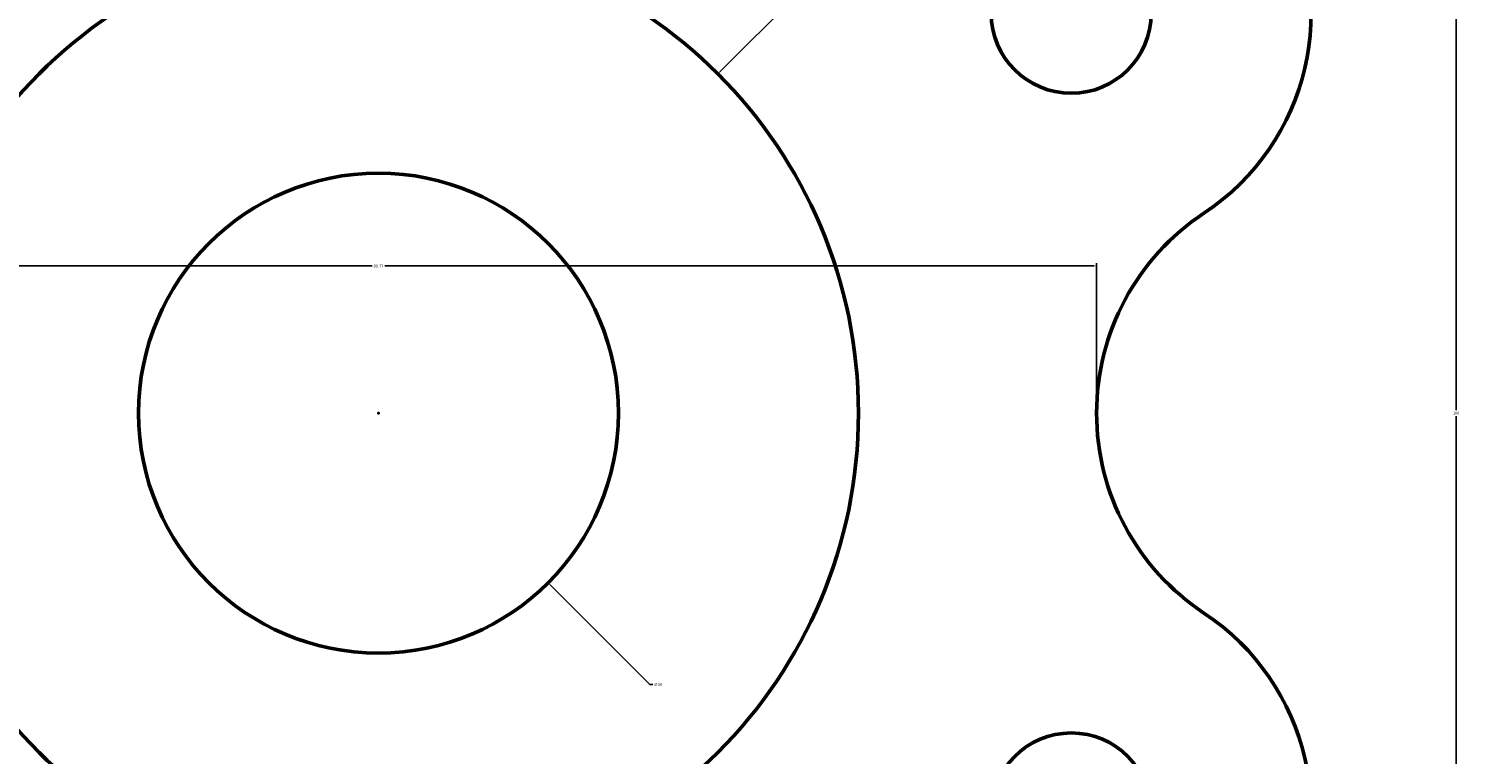
# Model space of a CAD drawing. Units: millimetres. Extents: x 2038 to 2173, y 1596 to 1745.
# Tile 3 of 4: x 2084 to 2173, y 1649 to 1695. Entities that reach past the tile are written whole.
import ezdxf

# ---------------------------------------------------------------- set-up
doc = ezdxf.new("R2010")
doc.units = ezdxf.units.MM
doc.layers.add('M-DIMS', color=2, linetype='Continuous', lineweight=18)
doc.layers.add('M-OUTL', color=7, linetype='Continuous', lineweight=50)
doc.styles.get("Standard").update_dxf_attribs({"font": 'arial.ttf'})
doc.dimstyles.get("Standard").update_dxf_attribs({"dimtxt": 0.18, "dimasz": 0.18, "dimexe": 0.18, "dimexo": 0.0625, "dimgap": 0.09, "dimtad": 0, "dimtih": 1, "dimtoh": 1, "dimdec": 4, "dimzin": 0, "dimdsep": 46, "dimtxsty": 'Standard', "dimcen": 0.09, "dimadec": 0, "dimazin": 0, "dimtfac": 1, "dimtdec": 4, "dimtofl": 0, "dimtmove": 0, "dimatfit": 3, "dimfxl": 1, "dimtolj": 1, "dimtzin": 0, "dimarcsym": 0})

# ---------------------------------------------------------------- blocks, each defined once
blk = doc.blocks.new('*U1')
blk.add_arc((-4.146, 7.965), 15, 243.55731, 356.44269)
blk = doc.blocks.new('*U2')
at = {"layer": 'M-OUTL', "color": 0, "linetype": 'ByBlock', "lineweight": -2, "transparency": 16777216, "rotation": 240}
blk.add_blockref('*U1', (2156.401, 1671.177), dxfattribs=at)
blk = doc.blocks.new('FLANGE-LUG-D10')
blk.add_circle((0, 0), 5)
blk.add_arc((0, 0), 15, 3.55731, 176.44269)
blk = doc.blocks.new('*D5')
at = {"layer": 'Defpoints', "color": 0, "transparency": 16777216}
for p in [(2038.131, 1735.784), (2105.488, 1735.784), (2105.488, 1605.784)]:
    blk.add_point(p, dxfattribs=at)
at = {"layer": 'M-DIMS', "color": 0, "lineweight": -2, "transparency": 16777216}
for p, q in [((2105.425, 1735.784), (2037.951, 1735.784)), ((2038.131, 1735.604), (2038.131, 1670.966)), ((2038.131, 1605.964), (2038.131, 1670.602)), ((2105.425, 1605.784), (2037.951, 1605.784))]:
    blk.add_line(p, q, dxfattribs=at)
at = {"layer": 'M-DIMS', "color": 0, "transparency": 16777216}
for points in [[(2038.101, 1735.604), (2038.161, 1735.604), (2038.131, 1735.784)], [(2038.101, 1605.964), (2038.161, 1605.964), (2038.131, 1605.784)]]:
    blk.add_solid(points, dxfattribs=at)
at = {"layer": 'M-DIMS', "color": 0, "transparency": 16777216, "insert": (2038.131, 1670.784), "char_height": 0.18, "attachment_point": 5}
blk.add_mtext('\\A1;130', dxfattribs=at)
blk = doc.blocks.new('*D6')
at = {"layer": 'Defpoints', "color": 0, "transparency": 16777216}
for p in [(2105.488, 1720.784), (2172.845, 1720.784), (2105.488, 1620.784)]:
    blk.add_point(p, dxfattribs=at)
at = {"layer": 'M-DIMS', "color": 0, "lineweight": -2, "transparency": 16777216}
for p, q in [((2105.55, 1720.784), (2173.025, 1720.784)), ((2172.845, 1720.604), (2172.845, 1670.966)), ((2172.845, 1620.964), (2172.845, 1670.602)), ((2105.55, 1620.784), (2173.025, 1620.784))]:
    blk.add_line(p, q, dxfattribs=at)
at = {"layer": 'M-DIMS', "color": 0, "transparency": 16777216}
for points in [[(2172.815, 1720.604), (2172.875, 1720.604), (2172.845, 1720.784)], [(2172.815, 1620.964), (2172.875, 1620.964), (2172.845, 1620.784)]]:
    blk.add_solid(points, dxfattribs=at)
at = {"layer": 'M-DIMS', "color": 0, "transparency": 16777216, "insert": (2172.845, 1670.784), "char_height": 0.18, "attachment_point": 5}
blk.add_mtext('\\A1;100', dxfattribs=at)
blk = doc.blocks.new('*D9')
at = {"layer": 'Defpoints', "color": 0, "transparency": 16777216}
for p in [(2150.372, 1679.984), (2060.603, 1670.784), (2150.372, 1670.784)]:
    blk.add_point(p, dxfattribs=at)
at = {"layer": 'M-DIMS', "color": 0, "lineweight": -2, "transparency": 16777216}
for p, q in [((2060.603, 1670.847), (2060.603, 1680.164)), ((2060.783, 1679.984), (2105.094, 1679.984)), ((2150.192, 1679.984), (2105.882, 1679.984)), ((2150.372, 1670.847), (2150.372, 1680.164))]:
    blk.add_line(p, q, dxfattribs=at)
at = {"layer": 'M-DIMS', "color": 0, "transparency": 16777216}
for points in [[(2060.783, 1680.014), (2060.783, 1679.954), (2060.603, 1679.984)], [(2150.192, 1680.014), (2150.192, 1679.954), (2150.372, 1679.984)]]:
    blk.add_solid(points, dxfattribs=at)
at = {"layer": 'M-DIMS', "color": 0, "transparency": 16777216, "insert": (2105.488, 1679.984), "char_height": 0.18, "attachment_point": 5}
blk.add_mtext('\\A1;89.77', dxfattribs=at)
blk = doc.blocks.new('*D10')
at = {"layer": 'Defpoints', "color": 0, "transparency": 16777216}
for p in [(2094.881, 1681.391), (2116.094, 1660.178)]:
    blk.add_point(p, dxfattribs=at)
at = {"layer": 'M-DIMS', "color": 0, "lineweight": -2, "transparency": 16777216}
for p, q in [((2105.398, 1670.784), (2105.578, 1670.784)), ((2105.488, 1670.694), (2105.488, 1670.874)), ((2122.458, 1653.814), (2116.222, 1660.05)), ((2122.638, 1653.814), (2122.458, 1653.814))]:
    blk.add_line(p, q, dxfattribs=at)
at = {"layer": 'M-DIMS', "color": 0, "transparency": 16777216}
blk.add_solid([(2116.243, 1660.072), (2116.2, 1660.029), (2116.094, 1660.178)], dxfattribs=at)
at = {"layer": 'M-DIMS', "color": 0, "transparency": 16777216, "insert": (2122.955, 1653.814), "char_height": 0.18, "attachment_point": 5}
blk.add_mtext('\\A1;∅30', dxfattribs=at)
blk = doc.blocks.new('*D11')
at = {"layer": 'Defpoints', "color": 0, "transparency": 16777216}
for p in [(2126.701, 1691.998), (2084.275, 1649.571)]:
    blk.add_point(p, dxfattribs=at)
at = {"layer": 'M-DIMS', "color": 0, "lineweight": -2, "transparency": 16777216}
for p, q in [((2139.428, 1704.726), (2126.828, 1692.125)), ((2139.608, 1704.726), (2139.428, 1704.726)), ((2105.398, 1670.784), (2105.578, 1670.784)), ((2105.488, 1670.694), (2105.488, 1670.874))]:
    blk.add_line(p, q, dxfattribs=at)
at = {"layer": 'M-DIMS', "color": 0, "transparency": 16777216}
blk.add_solid([(2126.807, 1692.146), (2126.849, 1692.104), (2126.701, 1691.998)], dxfattribs=at)
at = {"layer": 'M-DIMS', "color": 0, "transparency": 16777216, "insert": (2139.925, 1704.726), "char_height": 0.18, "attachment_point": 5}
blk.add_mtext('\\A1;∅60', dxfattribs=at)

msp = doc.modelspace()

# ---------------------------------------------------------------- linework, layer by layer
at = {"layer": 'M-OUTL'}
for radius in [30, 15]:
    msp.add_circle((2105.488, 1670.784), radius, dxfattribs=at)

# ---------------------------------------------------------------- block references
msp.add_blockref('*U2', (0, 0), dxfattribs=at)
for p, rotation in [((2148.789, 1695.784), 299.9999999999998), ((2148.789, 1645.784), 239.9999999999991)]:
    msp.add_blockref('FLANGE-LUG-D10', p, dxfattribs=dict(at, rotation=rotation))

# ---------------------------------------------------------------- dimensions: what is measured, and where the dimension line sits
at = {"layer": 'M-DIMS'}
for base, p1, p2, picture, middle in [((2038.131, 1735.784), (2105.488, 1605.784), (2105.488, 1735.784), '*D5', (2038.131, 1670.784)), ((2172.845, 1720.784), (2105.488, 1620.784), (2105.488, 1720.784), '*D6', (2172.845, 1670.784))]:
    dim = msp.add_linear_dim(base=base, p1=p1, p2=p2, angle=90, dimstyle='Standard', override={"dimdec": 0, "dimlfac": 1, "dimrnd": 0, "dimzin": 0, "dimdsep": 46, "dimlunit": 2}, dxfattribs=at)
    dim.commit()
    dim.dimension.update_dxf_attribs({"geometry": picture, "text_midpoint": middle})
for p1, p2, picture, middle in [((2084.275, 1649.571), (2126.701, 1691.998), '*D11', (2139.925, 1704.726)), ((2094.881, 1681.391), (2116.094, 1660.178), '*D10', (2122.955, 1653.814))]:
    dim = msp.add_diameter_dim_2p(p1=p1, p2=p2, dimstyle='Standard', override={"dimdec": 0, "dimlfac": 1, "dimrnd": 0, "dimzin": 0, "dimdsep": 46, "dimlunit": 2}, dxfattribs=at)
    dim.commit()
    dim.dimension.update_dxf_attribs({"geometry": picture, "text_midpoint": middle, "dimtype": 163})
dim = msp.add_linear_dim(base=(2150.372, 1679.984), p1=(2060.603, 1670.784), p2=(2150.372, 1670.784), dimstyle='Standard', override={"dimdec": 2, "dimlfac": 1, "dimrnd": 0, "dimzin": 0, "dimdsep": 46, "dimlunit": 2}, dxfattribs=at)
dim.commit()
dim.dimension.update_dxf_attribs({"geometry": '*D9', "text_midpoint": (2105.488, 1679.984)})

doc.saveas('drawing.dxf')
